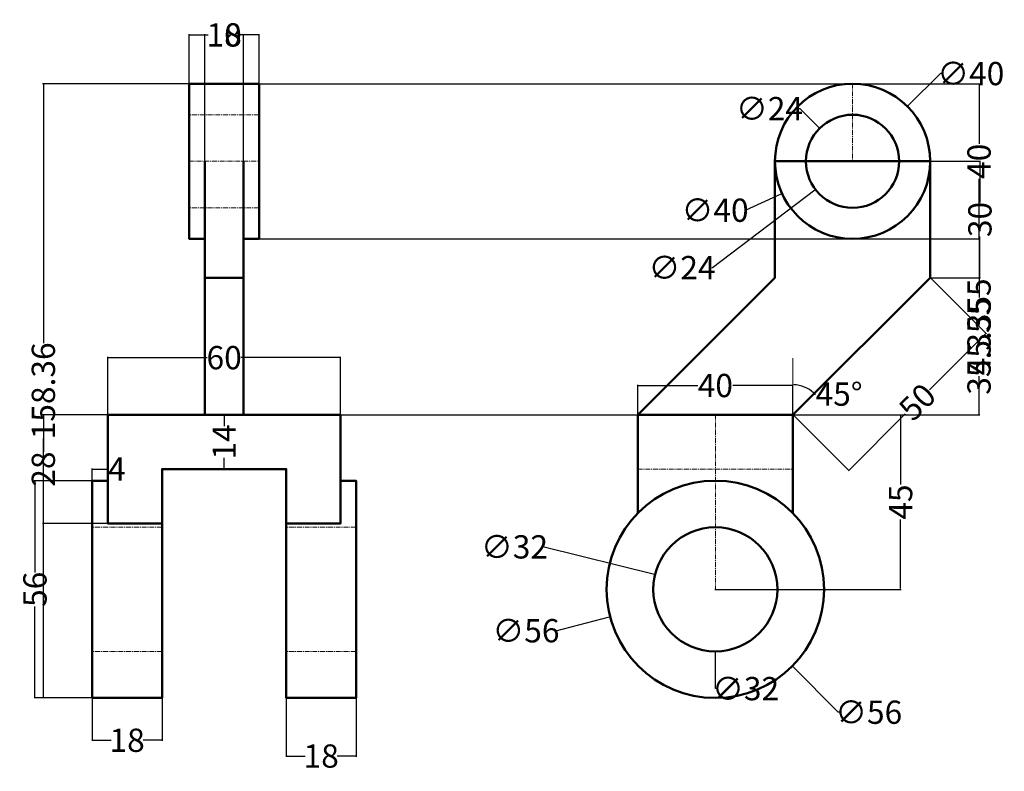
# Model space of a CAD drawing. Units: millimetres. Extents: x -19 to 235, y -89 to 104.
import ezdxf

# ---------------------------------------------------------------- set-up
doc = ezdxf.new("R2010")
doc.units = ezdxf.units.MM
doc.header["$MEASUREMENT"] = 0
doc.linetypes.add('CENTER', pattern=[2, 1.25, -0.25, 0.25, -0.25])
for name, color, linetype, lineweight in [('M-CNTR', 4, 'CENTER', 18), ('M-CONS', 8, 'Continuous', 13), ('M-DIMS', 2, 'Continuous', 25), ('M-OUTL', 7, 'Continuous', 50)]:
    doc.layers.add(name, color=color, linetype=linetype, lineweight=lineweight)
doc.styles.get("Standard").update_dxf_attribs({"font": 'arial.ttf'})
doc.dimstyles.get("Standard").update_dxf_attribs({"dimtxt": 6, "dimasz": 0.18, "dimexe": 0.18, "dimexo": 0.0625, "dimgap": 0.09, "dimtad": 0, "dimtoh": 1, "dimdec": 0, "dimzin": 0, "dimdsep": 46, "dimtxsty": 'Standard', "dimcen": 0.09, "dimadec": 0, "dimazin": 0, "dimtfac": 1, "dimtdec": 0, "dimtofl": 0, "dimtmove": 0, "dimatfit": 3, "dimfxl": 1, "dimtolj": 1, "dimtzin": 0, "dimarcsym": 0})

# ---------------------------------------------------------------- blocks, each defined once
blk = doc.blocks.new('*D1')
at = {"layer": 'Defpoints', "color": 0, "transparency": 16777216}
for p in [(63.65, 17.3), (3.65, 2.57), (63.65, 2.57)]:
    blk.add_point(p, dxfattribs=at)
at = {"layer": 'M-DIMS', "color": 0, "lineweight": -2, "transparency": 16777216}
for p, q in [((3.65, 2.63), (3.65, 17.48)), ((3.83, 17.3), (29.26, 17.3)), ((63.47, 17.3), (38.04, 17.3)), ((63.65, 2.63), (63.65, 17.48))]:
    blk.add_line(p, q, dxfattribs=at)
at = {"layer": 'M-DIMS', "color": 0, "transparency": 16777216}
for points in [[(3.83, 17.33), (3.83, 17.27), (3.65, 17.3)], [(63.47, 17.33), (63.47, 17.27), (63.65, 17.3)]]:
    blk.add_solid(points, dxfattribs=at)
at = {"layer": 'M-DIMS', "color": 0, "transparency": 16777216, "insert": (33.65, 17.3), "char_height": 6, "attachment_point": 5}
blk.add_mtext('\\A1;60', dxfattribs=at)
blk = doc.blocks.new('*D2')
at = {"layer": 'Defpoints', "color": 0, "transparency": 16777216}
for p in [(33.65, 2.57), (33.65, -11.43), (33.65, -11.43)]:
    blk.add_point(p, dxfattribs=at)
at = {"layer": 'M-DIMS', "color": 0, "lineweight": -2, "transparency": 16777216}
for p, q in [((33.59, 2.57), (33.47, 2.57)), ((33.65, 2.39), (33.65, -0.34)), ((33.65, -11.25), (33.65, -8.53)), ((33.59, -11.43), (33.47, -11.43))]:
    blk.add_line(p, q, dxfattribs=at)
at = {"layer": 'M-DIMS', "color": 0, "transparency": 16777216}
for points in [[(33.62, 2.39), (33.68, 2.39), (33.65, 2.57)], [(33.62, -11.25), (33.68, -11.25), (33.65, -11.43)]]:
    blk.add_solid(points, dxfattribs=at)
at = {"layer": 'M-DIMS', "color": 0, "transparency": 16777216, "insert": (33.65, -4.43), "char_height": 6, "attachment_point": 5, "rotation": 90}
blk.add_mtext('\\A1;14', dxfattribs=at)
blk = doc.blocks.new('*D3')
at = {"layer": 'Defpoints', "color": 0, "transparency": 16777216}
for p in [(3.65, -11.43), (-0.35, -14.43), (3.65, -14.43)]:
    blk.add_point(p, dxfattribs=at)
at = {"layer": 'M-DIMS', "color": 0, "lineweight": -2, "transparency": 16777216}
for p, q in [((-0.35, -14.37), (-0.35, -11.25)), ((-0.17, -11.43), (3.47, -11.43)), ((3.65, -14.37), (3.65, -11.25)), ((3.65, -11.43), (3.83, -11.43))]:
    blk.add_line(p, q, dxfattribs=at)
at = {"layer": 'M-DIMS', "color": 0, "transparency": 16777216}
for points in [[(-0.17, -11.4), (-0.17, -11.46), (-0.35, -11.43)], [(3.47, -11.4), (3.47, -11.46), (3.65, -11.43)]]:
    blk.add_solid(points, dxfattribs=at)
at = {"layer": 'M-DIMS', "color": 0, "transparency": 16777216, "insert": (5.99, -11.43), "char_height": 6, "attachment_point": 5}
blk.add_mtext('\\A1;4', dxfattribs=at)
blk = doc.blocks.new('*D4')
at = {"layer": 'Defpoints', "color": 0, "transparency": 16777216}
for p in [(-0.35, -14.43), (-15.09, -70.43), (-0.35, -70.43)]:
    blk.add_point(p, dxfattribs=at)
at = {"layer": 'M-DIMS', "color": 0, "lineweight": -2, "transparency": 16777216}
for p, q in [((-0.41, -14.43), (-15.27, -14.43)), ((-15.09, -14.61), (-15.09, -38.05)), ((-15.09, -70.25), (-15.09, -46.82)), ((-0.41, -70.43), (-15.27, -70.43))]:
    blk.add_line(p, q, dxfattribs=at)
at = {"layer": 'M-DIMS', "color": 0, "transparency": 16777216}
for points in [[(-15.12, -14.61), (-15.06, -14.61), (-15.09, -14.43)], [(-15.12, -70.25), (-15.06, -70.25), (-15.09, -70.43)]]:
    blk.add_solid(points, dxfattribs=at)
at = {"layer": 'M-DIMS', "color": 0, "transparency": 16777216, "insert": (-15.09, -42.43), "char_height": 6, "attachment_point": 5, "rotation": 90}
blk.add_mtext('\\A1;56', dxfattribs=at)
blk = doc.blocks.new('*D5')
at = {"layer": 'Defpoints', "color": 0, "transparency": 16777216}
for p in [(-0.35, -70.43), (17.65, -70.43), (17.65, -81.34)]:
    blk.add_point(p, dxfattribs=at)
at = {"layer": 'M-DIMS', "color": 0, "lineweight": -2, "transparency": 16777216}
for p, q in [((-0.35, -70.5), (-0.35, -81.52)), ((17.65, -70.5), (17.65, -81.52)), ((-0.17, -81.34), (4.54, -81.34)), ((17.47, -81.34), (12.76, -81.34))]:
    blk.add_line(p, q, dxfattribs=at)
at = {"layer": 'M-DIMS', "color": 0, "transparency": 16777216}
for points in [[(-0.17, -81.31), (-0.17, -81.37), (-0.35, -81.34)], [(17.47, -81.31), (17.47, -81.37), (17.65, -81.34)]]:
    blk.add_solid(points, dxfattribs=at)
at = {"layer": 'M-DIMS', "color": 0, "transparency": 16777216, "insert": (8.65, -81.34), "char_height": 6, "attachment_point": 5}
blk.add_mtext('\\A1;18', dxfattribs=at)
blk = doc.blocks.new('*D6')
at = {"layer": 'Defpoints', "color": 0, "transparency": 16777216}
for p in [(49.65, -70.43), (67.65, -70.43), (67.65, -85.41)]:
    blk.add_point(p, dxfattribs=at)
at = {"layer": 'M-DIMS', "color": 0, "lineweight": -2, "transparency": 16777216}
for p, q in [((49.65, -70.5), (49.65, -85.59)), ((67.65, -70.5), (67.65, -85.59)), ((49.83, -85.41), (54.54, -85.41)), ((67.47, -85.41), (62.76, -85.41))]:
    blk.add_line(p, q, dxfattribs=at)
at = {"layer": 'M-DIMS', "color": 0, "transparency": 16777216}
for points in [[(49.83, -85.38), (49.83, -85.44), (49.65, -85.41)], [(67.47, -85.38), (67.47, -85.44), (67.65, -85.41)]]:
    blk.add_solid(points, dxfattribs=at)
at = {"layer": 'M-DIMS', "color": 0, "transparency": 16777216, "insert": (58.65, -85.41), "char_height": 6, "attachment_point": 5}
blk.add_mtext('\\A1;18', dxfattribs=at)
blk = doc.blocks.new('*D7')
at = {"layer": 'Defpoints', "color": 0, "transparency": 16777216}
for p in [(215.55, 37.92), (180.19, 17.2), (182.19, 10.04), (180.19, 2.57), (180.19, 2.57)]:
    blk.add_point(p, dxfattribs=at)
at = {"layer": 'M-DIMS', "color": 0, "lineweight": -2, "transparency": 16777216}
blk.add_line((185.79, 7.91), (185.97, 7.91), dxfattribs=at)
for start, end in [(46.3328, 88.6672), (43.6672, 45)]:
    blk.add_arc((180.19, 2.57), 7.74, start, end, dxfattribs=at)
at = {"layer": 'M-DIMS', "color": 0, "transparency": 16777216}
for points in [[(180.37, 10.27), (180.37, 10.33), (180.19, 10.3)], [(185.55, 8.19), (185.51, 8.14), (185.66, 8.04)]]:
    blk.add_solid(points, dxfattribs=at)
at = {"layer": 'M-DIMS', "color": 0, "transparency": 16777216, "insert": (192.06, 7.91), "char_height": 6, "attachment_point": 5}
blk.add_mtext('\\A1;45°', dxfattribs=at)
blk = doc.blocks.new('*D8')
at = {"layer": 'Defpoints', "color": 0, "transparency": 16777216}
for p in [(180.19, 10.12), (140.19, 2.57), (180.19, 2.57)]:
    blk.add_point(p, dxfattribs=at)
at = {"layer": 'M-DIMS', "color": 0, "lineweight": -2, "transparency": 16777216}
for p, q in [((140.19, 2.63), (140.19, 10.3)), ((180.19, 2.63), (180.19, 10.3)), ((140.37, 10.12), (155.69, 10.12)), ((180.01, 10.12), (164.69, 10.12))]:
    blk.add_line(p, q, dxfattribs=at)
at = {"layer": 'M-DIMS', "color": 0, "transparency": 16777216}
for points in [[(140.37, 10.15), (140.37, 10.09), (140.19, 10.12)], [(180.01, 10.15), (180.01, 10.09), (180.19, 10.12)]]:
    blk.add_solid(points, dxfattribs=at)
at = {"layer": 'M-DIMS', "color": 0, "transparency": 16777216, "insert": (160.19, 10.12), "char_height": 6, "attachment_point": 5}
blk.add_mtext('\\A1;40', dxfattribs=at)
blk = doc.blocks.new('*D9')
at = {"layer": 'Defpoints', "color": 0, "transparency": 16777216}
for p in [(215.55, 37.92), (229.9, 23.56), (180.19, 2.57)]:
    blk.add_point(p, dxfattribs=at)
at = {"layer": 'M-DIMS', "color": 0, "lineweight": -2, "transparency": 16777216}
for p, q in [((215.59, 37.88), (230.03, 23.43)), ((229.78, 23.43), (215.32, 8.98)), ((194.68, -11.67), (209.13, 2.79)), ((180.23, 2.52), (194.68, -11.92))]:
    blk.add_line(p, q, dxfattribs=at)
at = {"layer": 'M-DIMS', "color": 0, "transparency": 16777216}
for points in [[(229.76, 23.46), (229.8, 23.41), (229.9, 23.56)], [(194.66, -11.64), (194.7, -11.69), (194.55, -11.79)]]:
    blk.add_solid(points, dxfattribs=at)
at = {"layer": 'M-DIMS', "color": 0, "transparency": 16777216, "insert": (212.23, 5.88), "char_height": 6, "attachment_point": 5, "rotation": 45}
blk.add_mtext('\\A1;50', dxfattribs=at)
blk = doc.blocks.new('*D10')
at = {"layer": 'Defpoints', "color": 0, "transparency": 16777216}
for p in [(215.55, 67.92), (215.55, 37.92), (228.35, 37.92)]:
    blk.add_point(p, dxfattribs=at)
at = {"layer": 'M-DIMS', "color": 0, "lineweight": -2, "transparency": 16777216}
for p, q in [((215.61, 67.92), (228.53, 67.92)), ((228.35, 67.74), (228.35, 57.3)), ((228.35, 38.1), (228.35, 48.55)), ((215.61, 37.92), (228.53, 37.92))]:
    blk.add_line(p, q, dxfattribs=at)
at = {"layer": 'M-DIMS', "color": 0, "transparency": 16777216}
for points in [[(228.32, 67.74), (228.38, 67.74), (228.35, 67.92)], [(228.32, 38.1), (228.38, 38.1), (228.35, 37.92)]]:
    blk.add_solid(points, dxfattribs=at)
at = {"layer": 'M-DIMS', "color": 0, "transparency": 16777216, "insert": (228.35, 52.92), "char_height": 6, "attachment_point": 5, "rotation": 90}
blk.add_mtext('\\A1;30', dxfattribs=at)
blk = doc.blocks.new('*D11')
at = {"layer": 'Defpoints', "color": 0, "transparency": 16777216}
for p in [(213.73, 76.24), (177.36, 59.61)]:
    blk.add_point(p, dxfattribs=at)
at = {"layer": 'M-DIMS', "color": 0, "lineweight": -2, "transparency": 16777216}
for p, q in [((195.46, 67.92), (195.64, 67.92)), ((195.55, 67.83), (195.55, 68.01)), ((167.96, 55.31), (177.19, 59.53)), ((167.78, 55.31), (167.96, 55.31))]:
    blk.add_line(p, q, dxfattribs=at)
at = {"layer": 'M-DIMS', "color": 0, "transparency": 16777216}
blk.add_solid([(177.18, 59.56), (177.2, 59.5), (177.36, 59.61)], dxfattribs=at)
at = {"layer": 'M-DIMS', "color": 0, "transparency": 16777216, "insert": (160.14, 55.31), "char_height": 6, "attachment_point": 5}
blk.add_mtext('\\A1;∅40', dxfattribs=at)
blk = doc.blocks.new('*D12')
at = {"layer": 'Defpoints', "color": 0, "transparency": 16777216}
for p in [(205.1, 75.18), (185.99, 60.67)]:
    blk.add_point(p, dxfattribs=at)
at = {"layer": 'M-DIMS', "color": 0, "lineweight": -2, "transparency": 16777216}
for p, q in [((195.46, 67.92), (195.64, 67.92)), ((195.55, 67.83), (195.55, 68.01)), ((159.44, 40.51), (185.84, 60.56)), ((159.26, 40.51), (159.44, 40.51))]:
    blk.add_line(p, q, dxfattribs=at)
at = {"layer": 'M-DIMS', "color": 0, "transparency": 16777216}
blk.add_solid([(185.83, 60.58), (185.86, 60.53), (185.99, 60.67)], dxfattribs=at)
at = {"layer": 'M-DIMS', "color": 0, "transparency": 16777216, "insert": (151.62, 40.51), "char_height": 6, "attachment_point": 5}
blk.add_mtext('\\A1;∅24', dxfattribs=at)
blk = doc.blocks.new('*D13')
at = {"layer": 'Defpoints', "color": 0, "transparency": 16777216}
for p in [(160.19, 2.57), (160.19, -42.43), (207.91, -42.43)]:
    blk.add_point(p, dxfattribs=at)
at = {"layer": 'M-DIMS', "color": 0, "lineweight": -2, "transparency": 16777216}
for p, q in [((160.25, 2.57), (208.09, 2.57)), ((207.91, 2.39), (207.91, -15.4)), ((207.91, -42.25), (207.91, -24.46)), ((160.25, -42.43), (208.09, -42.43))]:
    blk.add_line(p, q, dxfattribs=at)
at = {"layer": 'M-DIMS', "color": 0, "transparency": 16777216}
for points in [[(207.88, 2.39), (207.94, 2.39), (207.91, 2.57)], [(207.88, -42.25), (207.94, -42.25), (207.91, -42.43)]]:
    blk.add_solid(points, dxfattribs=at)
at = {"layer": 'M-DIMS', "color": 0, "transparency": 16777216, "insert": (207.91, -19.93), "char_height": 6, "attachment_point": 5, "rotation": 90}
blk.add_mtext('\\A1;45', dxfattribs=at)
blk = doc.blocks.new('*D14')
at = {"layer": 'Defpoints', "color": 0, "transparency": 16777216}
for p in [(187.29, -35.4), (133.09, -49.46)]:
    blk.add_point(p, dxfattribs=at)
at = {"layer": 'M-DIMS', "color": 0, "lineweight": -2, "transparency": 16777216}
for p, q in [((160.1, -42.43), (160.28, -42.43)), ((160.19, -42.52), (160.19, -42.34)), ((119.06, -53.1), (132.91, -49.51))]:
    blk.add_line(p, q, dxfattribs=at)
at = {"layer": 'M-DIMS', "color": 0, "transparency": 16777216}
blk.add_solid([(132.91, -49.48), (132.92, -49.54), (133.09, -49.46)], dxfattribs=at)
at = {"layer": 'M-DIMS', "color": 0, "transparency": 16777216, "insert": (111.41, -53.1), "char_height": 6, "attachment_point": 5}
blk.add_mtext('\\A1;∅56', dxfattribs=at)
blk = doc.blocks.new('*D15')
at = {"layer": 'Defpoints', "color": 0, "transparency": 16777216}
for p in [(144.66, -38.58), (175.72, -46.29)]:
    blk.add_point(p, dxfattribs=at)
at = {"layer": 'M-DIMS', "color": 0, "lineweight": -2, "transparency": 16777216}
for p, q in [((116.07, -31.48), (144.49, -38.54)), ((160.1, -42.43), (160.28, -42.43)), ((160.19, -42.52), (160.19, -42.34))]:
    blk.add_line(p, q, dxfattribs=at)
at = {"layer": 'M-DIMS', "color": 0, "transparency": 16777216}
blk.add_solid([(144.49, -38.51), (144.48, -38.56), (144.66, -38.58)], dxfattribs=at)
at = {"layer": 'M-DIMS', "color": 0, "transparency": 16777216, "insert": (108.45, -31.48), "char_height": 6, "attachment_point": 5}
blk.add_mtext('\\A1;∅32', dxfattribs=at)
blk = doc.blocks.new('*D16')
at = {"layer": 'Defpoints', "color": 0, "transparency": 16777216}
for p in [(-12.93, 87.92), (24.65, 87.92), (-0.35, -70.43)]:
    blk.add_point(p, dxfattribs=at)
at = {"layer": 'M-DIMS', "color": 0, "lineweight": -2, "transparency": 16777216}
for p, q in [((24.59, 87.92), (-13.11, 87.92)), ((-12.93, 87.74), (-12.93, 21)), ((-12.93, -70.25), (-12.93, -3.52)), ((-0.41, -70.43), (-13.11, -70.43))]:
    blk.add_line(p, q, dxfattribs=at)
at = {"layer": 'M-DIMS', "color": 0, "transparency": 16777216}
for points in [[(-12.96, 87.74), (-12.9, 87.74), (-12.93, 87.92)], [(-12.96, -70.25), (-12.9, -70.25), (-12.93, -70.43)]]:
    blk.add_solid(points, dxfattribs=at)
at = {"layer": 'M-DIMS', "color": 0, "transparency": 16777216, "insert": (-12.93, 8.74), "char_height": 6, "attachment_point": 5, "rotation": 90}
blk.add_mtext('\\A1;158.36', dxfattribs=at)
blk = doc.blocks.new('*D17')
at = {"layer": 'Defpoints', "color": 0, "transparency": 16777216}
for p in [(42.65, 100.5), (24.65, 87.92), (42.65, 87.92)]:
    blk.add_point(p, dxfattribs=at)
at = {"layer": 'M-DIMS', "color": 0, "lineweight": -2, "transparency": 16777216}
for p, q in [((24.65, 87.98), (24.65, 100.68)), ((24.83, 100.5), (29.54, 100.5)), ((42.47, 100.5), (37.76, 100.5)), ((42.65, 87.98), (42.65, 100.68))]:
    blk.add_line(p, q, dxfattribs=at)
at = {"layer": 'M-DIMS', "color": 0, "transparency": 16777216}
for points in [[(24.83, 100.53), (24.83, 100.47), (24.65, 100.5)], [(42.47, 100.53), (42.47, 100.47), (42.65, 100.5)]]:
    blk.add_solid(points, dxfattribs=at)
at = {"layer": 'M-DIMS', "color": 0, "transparency": 16777216, "insert": (33.65, 100.5), "char_height": 6, "attachment_point": 5}
blk.add_mtext('\\A1;18', dxfattribs=at)
blk = doc.blocks.new('*D18')
at = {"layer": 'Defpoints', "color": 0, "transparency": 16777216}
for p in [(38.65, 100.5), (28.65, 67.92), (38.65, 67.92)]:
    blk.add_point(p, dxfattribs=at)
at = {"layer": 'M-DIMS', "color": 0, "lineweight": -2, "transparency": 16777216}
for p, q in [((28.65, 67.98), (28.65, 100.68)), ((28.83, 100.5), (29.55, 100.5)), ((38.47, 100.5), (37.74, 100.5)), ((38.65, 67.98), (38.65, 100.68))]:
    blk.add_line(p, q, dxfattribs=at)
at = {"layer": 'M-DIMS', "color": 0, "transparency": 16777216}
for points in [[(28.83, 100.53), (28.83, 100.47), (28.65, 100.5)], [(38.47, 100.53), (38.47, 100.47), (38.65, 100.5)]]:
    blk.add_solid(points, dxfattribs=at)
at = {"layer": 'M-DIMS', "color": 0, "transparency": 16777216, "insert": (33.65, 100.5), "char_height": 6, "attachment_point": 5}
blk.add_mtext('\\A1;10', dxfattribs=at)
blk = doc.blocks.new('*D19')
at = {"layer": 'Defpoints', "color": 0, "transparency": 16777216}
for p in [(42.65, 87.92), (42.65, 47.92), (228.12, 47.92)]:
    blk.add_point(p, dxfattribs=at)
at = {"layer": 'M-DIMS', "color": 0, "lineweight": -2, "transparency": 16777216}
for p, q in [((42.71, 87.92), (228.3, 87.92)), ((228.12, 87.74), (228.12, 72.42)), ((228.12, 48.1), (228.12, 63.42)), ((42.71, 47.92), (228.3, 47.92))]:
    blk.add_line(p, q, dxfattribs=at)
at = {"layer": 'M-DIMS', "color": 0, "transparency": 16777216}
for points in [[(228.09, 87.74), (228.15, 87.74), (228.12, 87.92)], [(228.09, 48.1), (228.15, 48.1), (228.12, 47.92)]]:
    blk.add_solid(points, dxfattribs=at)
at = {"layer": 'M-DIMS', "color": 0, "transparency": 16777216, "insert": (228.12, 67.92), "char_height": 6, "attachment_point": 5, "rotation": 90}
blk.add_mtext('\\A1;40', dxfattribs=at)
blk = doc.blocks.new('*D20')
at = {"layer": 'Defpoints', "color": 0, "transparency": 16777216}
for p in [(42.65, 47.92), (228.12, 47.92), (38.65, 2.57)]:
    blk.add_point(p, dxfattribs=at)
at = {"layer": 'M-DIMS', "color": 0, "lineweight": -2, "transparency": 16777216}
for p, q in [((42.71, 47.92), (228.3, 47.92)), ((228.12, 47.74), (228.12, 37.93)), ((228.12, 2.75), (228.12, 12.56)), ((38.71, 2.57), (228.3, 2.57))]:
    blk.add_line(p, q, dxfattribs=at)
at = {"layer": 'M-DIMS', "color": 0, "transparency": 16777216}
for points in [[(228.09, 47.74), (228.15, 47.74), (228.12, 47.92)], [(228.09, 2.75), (228.15, 2.75), (228.12, 2.57)]]:
    blk.add_solid(points, dxfattribs=at)
at = {"layer": 'M-DIMS', "color": 0, "transparency": 16777216, "insert": (228.12, 25.24), "char_height": 6, "attachment_point": 5, "rotation": 90}
blk.add_mtext('\\A1;45.355', dxfattribs=at)
blk = doc.blocks.new('*D21')
at = {"layer": 'Defpoints', "color": 0, "transparency": 16777216}
for p in [(3.65, 2.57), (-12.93, -25.43), (3.65, -25.43)]:
    blk.add_point(p, dxfattribs=at)
at = {"layer": 'M-DIMS', "color": 0, "lineweight": -2, "transparency": 16777216}
for p, q in [((3.59, 2.57), (-13.11, 2.57)), ((-12.93, 2.39), (-12.93, -6.99)), ((-12.93, -25.25), (-12.93, -15.88)), ((3.59, -25.43), (-13.11, -25.43))]:
    blk.add_line(p, q, dxfattribs=at)
at = {"layer": 'M-DIMS', "color": 0, "transparency": 16777216}
for points in [[(-12.96, 2.39), (-12.9, 2.39), (-12.93, 2.57)], [(-12.96, -25.25), (-12.9, -25.25), (-12.93, -25.43)]]:
    blk.add_solid(points, dxfattribs=at)
at = {"layer": 'M-DIMS', "color": 0, "transparency": 16777216, "insert": (-12.93, -11.43), "char_height": 6, "attachment_point": 5, "rotation": 90}
blk.add_mtext('\\A1;28', dxfattribs=at)
blk = doc.blocks.new('*D22')
at = {"layer": 'Defpoints', "color": 0, "transparency": 16777216}
for p in [(215.55, 37.92), (180.19, 2.57), (228.12, 2.57)]:
    blk.add_point(p, dxfattribs=at)
at = {"layer": 'M-DIMS', "color": 0, "lineweight": -2, "transparency": 16777216}
for p, q in [((215.61, 37.92), (228.3, 37.92)), ((228.12, 37.74), (228.12, 32.81)), ((228.12, 2.75), (228.12, 7.68)), ((180.25, 2.57), (228.3, 2.57))]:
    blk.add_line(p, q, dxfattribs=at)
at = {"layer": 'M-DIMS', "color": 0, "transparency": 16777216}
for points in [[(228.09, 37.74), (228.15, 37.74), (228.12, 37.92)], [(228.09, 2.75), (228.15, 2.75), (228.12, 2.57)]]:
    blk.add_solid(points, dxfattribs=at)
at = {"layer": 'M-DIMS', "color": 0, "transparency": 16777216, "insert": (228.12, 20.24), "char_height": 6, "attachment_point": 5, "rotation": 90}
blk.add_mtext('\\A1;35.355', dxfattribs=at)
blk = doc.blocks.new('*D23')
at = {"layer": 'Defpoints', "color": 0, "transparency": 16777216}
for p in [(140.39, -22.64), (179.99, -62.23)]:
    blk.add_point(p, dxfattribs=at)
at = {"layer": 'M-DIMS', "color": 0, "lineweight": -2, "transparency": 16777216}
for p, q in [((160.1, -42.43), (160.28, -42.43)), ((160.19, -42.52), (160.19, -42.34)), ((191.87, -74.11), (180.12, -62.36)), ((192.05, -74.11), (191.87, -74.11))]:
    blk.add_line(p, q, dxfattribs=at)
at = {"layer": 'M-DIMS', "color": 0, "transparency": 16777216}
blk.add_solid([(180.14, -62.34), (180.1, -62.38), (179.99, -62.23)], dxfattribs=at)
at = {"layer": 'M-DIMS', "color": 0, "transparency": 16777216, "insert": (199.7, -74.11), "char_height": 6, "attachment_point": 5}
blk.add_mtext('\\A1;∅56', dxfattribs=at)
blk = doc.blocks.new('*D24')
at = {"layer": 'Defpoints', "color": 0, "transparency": 16777216}
for p in [(160.19, -26.43), (160.19, -58.43)]:
    blk.add_point(p, dxfattribs=at)
at = {"layer": 'M-DIMS', "color": 0, "lineweight": -2, "transparency": 16777216}
for p, q in [((160.1, -42.43), (160.28, -42.43)), ((160.19, -42.52), (160.19, -42.34)), ((160.19, -68.03), (160.19, -58.61)), ((160.37, -68.03), (160.19, -68.03))]:
    blk.add_line(p, q, dxfattribs=at)
at = {"layer": 'M-DIMS', "color": 0, "transparency": 16777216}
blk.add_solid([(160.22, -58.61), (160.16, -58.61), (160.19, -58.43)], dxfattribs=at)
at = {"layer": 'M-DIMS', "color": 0, "transparency": 16777216, "insert": (167.99, -68.03), "char_height": 6, "attachment_point": 5}
blk.add_mtext('\\A1;∅32', dxfattribs=at)
blk = doc.blocks.new('*D25')
at = {"layer": 'Defpoints', "color": 0, "transparency": 16777216}
for p in [(209.69, 82.06), (181.4, 53.78)]:
    blk.add_point(p, dxfattribs=at)
at = {"layer": 'M-DIMS', "color": 0, "lineweight": -2, "transparency": 16777216}
for p, q in [((218.18, 90.54), (209.82, 82.19)), ((218.36, 90.54), (218.18, 90.54)), ((195.46, 67.92), (195.64, 67.92)), ((195.55, 67.83), (195.55, 68.01))]:
    blk.add_line(p, q, dxfattribs=at)
at = {"layer": 'M-DIMS', "color": 0, "transparency": 16777216}
blk.add_solid([(209.8, 82.21), (209.84, 82.17), (209.69, 82.06)], dxfattribs=at)
at = {"layer": 'M-DIMS', "color": 0, "transparency": 16777216, "insert": (226, 90.54), "char_height": 6, "attachment_point": 5}
blk.add_mtext('\\A1;∅40', dxfattribs=at)
blk = doc.blocks.new('*D26')
at = {"layer": 'Defpoints', "color": 0, "transparency": 16777216}
for p in [(187.06, 76.41), (204.03, 59.43)]:
    blk.add_point(p, dxfattribs=at)
at = {"layer": 'M-DIMS', "color": 0, "lineweight": -2, "transparency": 16777216}
for p, q in [((181.79, 81.5), (181.97, 81.5)), ((181.97, 81.5), (186.93, 76.54)), ((195.46, 67.92), (195.64, 67.92)), ((195.55, 67.83), (195.55, 68.01))]:
    blk.add_line(p, q, dxfattribs=at)
at = {"layer": 'M-DIMS', "color": 0, "transparency": 16777216}
blk.add_solid([(186.96, 76.56), (186.91, 76.51), (187.06, 76.41)], dxfattribs=at)
at = {"layer": 'M-DIMS', "color": 0, "transparency": 16777216, "insert": (174.15, 81.5), "char_height": 6, "attachment_point": 5}
blk.add_mtext('\\A1;∅24', dxfattribs=at)

msp = doc.modelspace()

# ---------------------------------------------------------------- linework, layer by layer
at = {"layer": 'M-CNTR'}
for p, q in [((195.5452, 87.9213), (195.5452, 67.9213)), ((42.6488, 79.9213), (24.6488, 79.9213)), ((24.5288, 67.9213), (42.6488, 67.9213)), ((42.6488, 55.9213), (24.6488, 55.9213)), ((160.1899, 2.5659), (160.1899, -42.4341)), ((140.1899, -11.4341), (180.1899, -11.4341)), ((160.1899, -14.4341), (160.1899, -14.4341)), ((17.6488, -26.4341), (-0.3512, -26.4341)), ((67.6488, -26.4341), (49.6488, -26.4341)), ((17.6488, -58.4341), (-0.3512, -58.4341)), ((67.6488, -58.4341), (49.6488, -58.4341))]:
    msp.add_line(p, q, dxfattribs=at)
at = {"layer": 'M-CONS'}
msp.add_line((180.1899, 2.5659), (180.1899, 17.2044), dxfattribs=at)
at = {"layer": 'M-OUTL'}
for points in [[(28.6488, 47.9213), (24.6488, 47.9213), (24.6488, 87.9213), (42.6488, 87.9213), (42.6488, 47.9213), (38.6488, 47.9213)], [(28.6488, 67.9213), (28.6488, 47.9213), (28.6488, 37.9213)], [(38.6488, 67.9213), (38.6488, 47.9213), (38.6488, 2.5659)], [(140.1899, 2.5659), (175.5452, 37.9213), (175.5452, 67.9213), (215.5452, 67.9213), (215.5452, 37.9213), (180.1899, 2.5659)], [(63.6488, -14.4341), (67.6488, -14.4341), (67.6488, -70.4341), (49.6488, -70.4341), (49.6488, -25.4341), (63.6488, -25.4341), (63.6488, 2.5659), (38.6488, 2.5659), (28.6488, 2.5659), (28.6488, 37.9213), (38.6488, 37.9213)], [(28.6488, 2.5659), (3.6488, 2.5659), (3.6488, -25.4341), (17.6488, -25.4341)], [(140.1899, -22.8381), (140.1899, 2.5659), (180.1899, 2.5659), (180.1899, -22.8381)], [(3.6488, -14.4341), (-0.3512, -14.4341), (-0.3512, -70.4341), (17.6488, -70.4341), (17.6488, -25.4341), (17.6488, -11.4341), (49.6488, -11.4341), (49.6488, -25.4341)]]:
    msp.add_lwpolyline(points, dxfattribs=at)
for centre, radius in [((195.5452, 67.9213), 20), ((195.5452, 67.9213), 12), ((160.1899, -42.4341), 28), ((160.1899, -42.4341), 16)]:
    msp.add_circle(centre, radius, dxfattribs=at)

# ---------------------------------------------------------------- dimensions: what is measured, and where the dimension line sits
at = {"layer": 'M-DIMS'}
for base, p1, p2, override, picture, middle in [((42.6488, 100.4963), (24.6488, 87.9213), (42.6488, 87.9213), {"dimdec": 0, "dimlfac": 1, "dimrnd": 0, "dimzin": 0, "dimdsep": 46, "dimlunit": 2}, '*D17', (33.6488, 100.4963)), ((38.6488, 100.4963), (28.6488, 67.9213), (38.6488, 67.9213), {"dimdec": 0, "dimlfac": 1, "dimrnd": 0, "dimzin": 0, "dimdsep": 46, "dimlunit": 2}, '*D18', (33.6488, 100.4963)), ((63.6488, 17.2999), (3.6488, 2.5659), (63.6488, 2.5659), {"dimclrd": 0, "dimclre": 0, "dimclrt": 0}, '*D1', (33.6488, 17.2999)), ((180.1899, 10.1234), (140.1899, 2.5659), (180.1899, 2.5659), {"dimclrd": 0, "dimclre": 0, "dimclrt": 0}, '*D8', (160.1899, 10.1234)), ((3.6488, -11.4341), (-0.3512, -14.4341), (3.6488, -14.4341), {"dimclrd": 0, "dimclre": 0, "dimclrt": 0}, '*D3', (5.9938, -11.4341)), ((17.6488, -81.3392), (-0.3512, -70.4341), (17.6488, -70.4341), {"dimclrd": 0, "dimclre": 0, "dimclrt": 0}, '*D5', (8.6488, -81.3392)), ((67.6488, -85.409), (49.6488, -70.4341), (67.6488, -70.4341), {"dimclrd": 0, "dimclre": 0, "dimclrt": 0}, '*D6', (58.6488, -85.409))]:
    dim = msp.add_linear_dim(base=base, p1=p1, p2=p2, dimstyle='Standard', override=override, dxfattribs=at)
    dim.commit()
    dim.dimension.update_dxf_attribs({"geometry": picture, "text_midpoint": middle})
for p1, p2, override, picture, middle in [((181.4, 53.7822), (209.6904, 82.0604), {"dimdec": 0, "dimlfac": 1, "dimrnd": 0, "dimzin": 0, "dimdsep": 46, "dimlunit": 2}, '*D25', (225.9986, 90.5438)), ((204.0287, 59.4342), (187.0617, 76.4083), {"dimdec": 0, "dimlfac": 1, "dimrnd": 0, "dimzin": 0, "dimdsep": 46, "dimlunit": 2}, '*D26', (174.1525, 81.5005)), ((213.7348, 76.2362), (177.3556, 59.6063), {"dimclrd": 0, "dimclre": 0, "dimclrt": 0}, '*D11', (160.1411, 55.3123)), ((205.1031, 75.1771), (185.9873, 60.6655), {"dimclrd": 0, "dimclre": 0, "dimclrt": 0}, '*D12', (151.6219, 40.5132)), ((140.3888, -22.6372), (179.991, -62.231), {"dimdec": 0, "dimlfac": 1, "dimrnd": 0, "dimzin": 0, "dimdsep": 46, "dimlunit": 2}, '*D23', (199.701, -74.1091)), ((175.7184, -46.2894), (144.6613, -38.5787), {"dimclrd": 0, "dimclre": 0, "dimclrt": 0}, '*D15', (116.0705, -31.4804)), ((160.1897, -26.4341), (160.19, -58.4341), {"dimdec": 0, "dimlfac": 1, "dimrnd": 0, "dimzin": 0, "dimdsep": 46, "dimlunit": 2}, '*D24', (167.9908, -68.0341)), ((187.293, -35.4039), (133.0868, -49.4642), {"dimclrd": 0, "dimclre": 0, "dimclrt": 0}, '*D14', (119.057, -53.1033))]:
    dim = msp.add_diameter_dim_2p(p1=p1, p2=p2, dimstyle='Standard', override=override, dxfattribs=at)
    dim.commit()
    dim.dimension.update_dxf_attribs({"geometry": picture, "text_midpoint": middle, "dimtype": 163})
for base, p1, p2, override, picture, middle in [((-12.9262, 87.9213), (-0.3512, -70.4341), (24.6488, 87.9213), {"dimdec": 2, "dimlfac": 1, "dimrnd": 0, "dimzin": 0, "dimdsep": 46, "dimlunit": 2}, '*D16', (-12.9262, 8.7436)), ((228.1202, 47.9213), (42.6488, 87.9213), (42.6488, 47.9213), {"dimdec": 0, "dimlfac": 1, "dimrnd": 0, "dimzin": 0, "dimdsep": 46, "dimlunit": 2}, '*D19', (228.1202, 67.9213)), ((228.3518, 37.9213), (215.5452, 67.9213), (215.5452, 37.9213), {"dimclrd": 0, "dimclre": 0, "dimclrt": 0}, '*D10', (228.3518, 52.9213)), ((228.1202, 47.9213), (38.6488, 2.5659), (42.6488, 47.9213), {"dimdec": 3, "dimlfac": 1, "dimrnd": 0, "dimzin": 0, "dimdsep": 46, "dimlunit": 2}, '*D20', (228.1202, 25.2436)), ((228.1202, 2.5659), (215.5452, 37.9213), (180.1899, 2.5659), {"dimdec": 3, "dimlfac": 1, "dimrnd": 0, "dimzin": 0, "dimdsep": 46, "dimlunit": 2}, '*D22', (228.1202, 20.2436)), ((-12.9262, -25.4341), (3.6488, 2.5659), (3.6488, -25.4341), {"dimdec": 0, "dimlfac": 1, "dimrnd": 0, "dimzin": 0, "dimdsep": 46, "dimlunit": 2}, '*D21', (-12.9262, -11.4341)), ((33.6488, -11.4341), (33.6488, 2.5659), (33.6488, -11.4341), {"dimclrd": 0, "dimclre": 0, "dimclrt": 0}, '*D2', (33.6488, -4.4341)), ((207.9074, -42.4341), (160.1899, 2.5659), (160.1899, -42.4341), {"dimclrd": 0, "dimclre": 0, "dimclrt": 0}, '*D13', (207.9074, -19.9341)), ((-15.0882, -70.4341), (-0.3512, -14.4341), (-0.3512, -70.4341), {"dimclrd": 0, "dimclre": 0, "dimclrt": 0}, '*D4', (-15.0882, -42.4341))]:
    dim = msp.add_linear_dim(base=base, p1=p1, p2=p2, angle=90, dimstyle='Standard', override=override, dxfattribs=at)
    dim.commit()
    dim.dimension.update_dxf_attribs({"geometry": picture, "text_midpoint": middle})
dim = msp.add_angular_dim_2l(base=(182.1927, 10.0407), line1=((215.5452, 37.9213), (180.1899, 2.5659)), line2=((180.1899, 2.5659), (180.1899, 17.2044)), dimstyle='Standard', override={"dimclrd": 0, "dimclre": 0, "dimclrt": 0}, dxfattribs=at)
dim.commit()
dim.dimension.update_dxf_attribs({"geometry": '*D7', "text_midpoint": (192.0637, 7.9091)})
dim = msp.add_aligned_dim(p1=(180.1899, 2.5659), p2=(215.5452, 37.9213), distance=-20.3072, dimstyle='Standard', override={"dimclrd": 0, "dimclre": 0, "dimclrt": 0}, dxfattribs=at)
dim.commit()
dim.dimension.update_dxf_attribs({"geometry": '*D9', "text_midpoint": (212.2269, 5.8842)})

doc.saveas('drawing.dxf')
